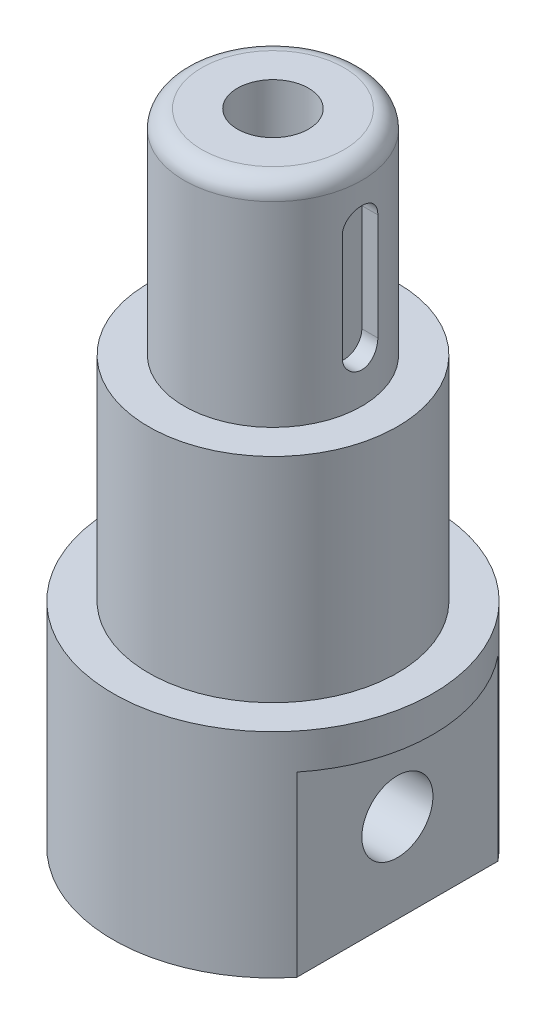
ISO-10303-21;
HEADER;
FILE_DESCRIPTION(('STEP AP214'),'2;1');
FILE_NAME('part.step','',(''),(''),'','','');
FILE_SCHEMA(('AUTOMOTIVE_DESIGN { 1 0 10303 214 1 1 1 1 }'));
ENDSEC;
DATA;
#1=APPLICATION_CONTEXT('core data for automotive mechanical design processes');
#2=APPLICATION_PROTOCOL_DEFINITION('international standard','automotive_design',2000,#1);
#3=PRODUCT_CONTEXT('',#1,'mechanical');
#4=PRODUCT('Part','Part','',(#3));
#5=PRODUCT_RELATED_PRODUCT_CATEGORY('part','',(#4));
#6=PRODUCT_DEFINITION_FORMATION('','',#4);
#7=PRODUCT_DEFINITION_CONTEXT('part definition',#1,'design');
#8=PRODUCT_DEFINITION('design','',#6,#7);
#9=PRODUCT_DEFINITION_SHAPE('','',#8);
#10=(LENGTH_UNIT() NAMED_UNIT(*) SI_UNIT(.MILLI.,.METRE.));
#11=(NAMED_UNIT(*) PLANE_ANGLE_UNIT() SI_UNIT($,.RADIAN.));
#12=(NAMED_UNIT(*) SI_UNIT($,.STERADIAN.) SOLID_ANGLE_UNIT());
#13=UNCERTAINTY_MEASURE_WITH_UNIT(LENGTH_MEASURE(1.E-05),#10,'distance_accuracy_value','');
#14=(GEOMETRIC_REPRESENTATION_CONTEXT(3) GLOBAL_UNCERTAINTY_ASSIGNED_CONTEXT((#13)) GLOBAL_UNIT_ASSIGNED_CONTEXT((#10,
#11,#12)) REPRESENTATION_CONTEXT('',''));
#15=CARTESIAN_POINT('',(0.,0.,0.));
#16=DIRECTION('',(0.,0.,1.));
#17=DIRECTION('',(1.,0.,0.));
#18=AXIS2_PLACEMENT_3D('',#15,#16,#17);
#19=CARTESIAN_POINT('',(0.,-40.6315789473685,0.));
#20=DIRECTION('',(0.,-1.,0.));
#21=DIRECTION('',(0.,0.,-1.));
#22=AXIS2_PLACEMENT_3D('',#19,#20,#21);
#23=CYLINDRICAL_SURFACE('',#22,9.99999999999998);
#24=CARTESIAN_POINT('',(-9.79795897113269,53.5481247085623,-2.));
#25=CARTESIAN_POINT('',(-9.79795611157837,53.4924575712637,-2.00000029709046));
#26=CARTESIAN_POINT('',(-9.7984339846543,53.4368176697574,-1.99767440405642));
#27=CARTESIAN_POINT('',(-9.8003213815013,53.3259472728948,-1.98839986829158));
#28=CARTESIAN_POINT('',(-9.80173079002195,53.2707167277472,-1.98145179742019));
#29=CARTESIAN_POINT('',(-9.80730283285148,53.1064148282608,-1.95376239954904));
#30=CARTESIAN_POINT('',(-9.81280956758552,52.9984618510279,-1.92617555297558));
#31=CARTESIAN_POINT('',(-9.82677660401679,52.7888395150785,-1.85359362042638));
#32=CARTESIAN_POINT('',(-9.83523723174862,52.6871708514489,-1.80859661275257));
#33=CARTESIAN_POINT('',(-9.85415440257655,52.4927949408026,-1.7025082088197));
#34=CARTESIAN_POINT('',(-9.86461115250624,52.4000886239446,-1.64141514447461));
#35=CARTESIAN_POINT('',(-9.88650550448303,52.2250050351923,-1.50396101869286));
#36=CARTESIAN_POINT('',(-9.89795377776162,52.1427721441036,-1.42741780364327));
#37=CARTESIAN_POINT('',(-9.92044851228357,51.9922158299872,-1.26162118198369));
#38=CARTESIAN_POINT('',(-9.9314949110525,51.9238945621014,-1.17236580968336));
#39=CARTESIAN_POINT('',(-9.9520562085508,51.8025469067149,-0.982720106800588));
#40=CARTESIAN_POINT('',(-9.96155694564012,51.7496587701377,-0.882239649549983));
#41=CARTESIAN_POINT('',(-9.97783510908993,51.6615729394628,-0.673602404217795));
#42=CARTESIAN_POINT('',(-9.98461293824418,51.6263726286505,-0.565446754297826));
#43=CARTESIAN_POINT('',(-9.99460635553982,51.5751106116245,-0.346034817774202));
#44=CARTESIAN_POINT('',(-9.99786765043074,51.5588031295946,-0.234838069151994));
#45=CARTESIAN_POINT('',(-10.0006184349224,51.5450227496855,-0.0112397534982628));
#46=CARTESIAN_POINT('',(-10.000108200481,51.5475484738055,0.101161724783846));
#47=CARTESIAN_POINT('',(-9.99540868887642,51.5711771093056,0.322284405513384));
#48=CARTESIAN_POINT('',(-9.99127193663418,51.5920148083719,0.43103522671446));
#49=CARTESIAN_POINT('',(-9.97984349003514,51.6512550625144,0.643464013108169));
#50=CARTESIAN_POINT('',(-9.97255169250399,51.6896581920068,0.747141812282547));
#51=CARTESIAN_POINT('',(-9.95554578241049,51.783185515553,0.94724054262592));
#52=CARTESIAN_POINT('',(-9.94581664782191,51.8384138824143,1.04361145363295));
#53=CARTESIAN_POINT('',(-9.92500903258343,51.9639452491157,1.22581287576612));
#54=CARTESIAN_POINT('',(-9.91393044014084,52.0342494982499,1.31164251244036));
#55=CARTESIAN_POINT('',(-9.89142074737008,52.1893814318128,1.47189241307715));
#56=CARTESIAN_POINT('',(-9.87998686483478,52.2744395127055,1.54608938999209));
#57=CARTESIAN_POINT('',(-9.85823412232846,52.4559342255401,1.6792217997989));
#58=CARTESIAN_POINT('',(-9.84791557170813,52.5523739988948,1.73815300484306));
#59=CARTESIAN_POINT('',(-9.82955460084641,52.7542295184542,1.83915990928954));
#60=CARTESIAN_POINT('',(-9.82151838996689,52.8596687553555,1.881189753269));
#61=CARTESIAN_POINT('',(-9.80872322124985,53.0762419710737,1.94681419465983));
#62=CARTESIAN_POINT('',(-9.80395938256573,53.1873672018586,1.97043625496866));
#63=CARTESIAN_POINT('',(-9.80006354383924,53.3408383422552,1.98966587624394));
#64=CARTESIAN_POINT('',(-9.79927519743984,53.3822329881272,1.99354251131102));
#65=CARTESIAN_POINT('',(-9.79822334773542,53.4651204368372,1.9987063293293));
#66=CARTESIAN_POINT('',(-9.79795896609648,53.5066129584739,1.99999784580931));
#67=CARTESIAN_POINT('',(-9.7979589711327,53.5481247085623,2.));
#68=B_SPLINE_CURVE_WITH_KNOTS('',3,(#24,#25,#26,#27,#28,#29,#30,#31,#32,#33,#34,#35,#36,#37,#38,
#39,#40,#41,#42,#43,#44,#45,#46,#47,#48,#49,#50,#51,#52,#53,#54,#55,#56,#57,#58,#59,#60,#61,#62,
#63,#64,#65,#66,#67),.UNSPECIFIED.,.F.,.F.,(4,2,2,2,2,2,2,2,2,2,2,2,2,2,2,2,2,2,2,2,2,4),(0.,
0.166897020715838,0.333773396643063,0.666722601037227,0.999708566174147,1.33272905329864,
1.66993288931439,2.00718892413592,2.34737937755194,2.68751948879679,3.02318320738907,
3.35882236614863,3.68967912555438,4.0205467052512,4.35350597112352,4.68649283901808,
5.02524540329293,5.3640916848566,5.70385119298729,6.04310283225105,6.16778801087552,
6.29226399953898),.UNSPECIFIED.);
#69=CARTESIAN_POINT('',(-9.79795897113269,53.5481247085623,-2.));
#70=VERTEX_POINT('',#69);
#71=CARTESIAN_POINT('',(-9.79795897113269,53.5481247085623,2.));
#72=VERTEX_POINT('',#71);
#73=EDGE_CURVE('E294',#70,#72,#68,.T.);
#74=ORIENTED_EDGE('',*,*,#73,.F.);
#75=DIRECTION('',(0.,-1.,0.));
#76=VECTOR('',#75,1.);
#77=CARTESIAN_POINT('',(-9.79795897113269,-40.6315789473685,-2.00000000000002));
#78=LINE('',#77,#76);
#79=CARTESIAN_POINT('',(-9.79795897113269,65.5481247085623,-2.));
#80=VERTEX_POINT('',#79);
#81=EDGE_CURVE('E11',#80,#70,#78,.T.);
#82=ORIENTED_EDGE('',*,*,#81,.F.);
#83=CARTESIAN_POINT('',(-9.79795897113269,65.5481247085623,2.));
#84=CARTESIAN_POINT('',(-9.79795611157837,65.603791845861,2.00000029709046));
#85=CARTESIAN_POINT('',(-9.7984339846543,65.6594317473673,1.99767440405642));
#86=CARTESIAN_POINT('',(-9.8003213815013,65.7703021442299,1.98839986829158));
#87=CARTESIAN_POINT('',(-9.80173079002195,65.8255326893775,1.98145179742019));
#88=CARTESIAN_POINT('',(-9.80730283285148,65.9898345888639,1.95376239954903));
#89=CARTESIAN_POINT('',(-9.81280956758552,66.0977875660968,1.92617555297558));
#90=CARTESIAN_POINT('',(-9.82677660401679,66.3074099020462,1.85359362042638));
#91=CARTESIAN_POINT('',(-9.83523723174862,66.4090785656758,1.80859661275257));
#92=CARTESIAN_POINT('',(-9.85415440257655,66.6034544763221,1.7025082088197));
#93=CARTESIAN_POINT('',(-9.86461115250624,66.6961607931801,1.64141514447462));
#94=CARTESIAN_POINT('',(-9.88650550448302,66.8712443819324,1.50396101869286));
#95=CARTESIAN_POINT('',(-9.89795377776162,66.9534772730211,1.42741780364328));
#96=CARTESIAN_POINT('',(-9.92044851228357,67.1040335871375,1.2616211819837));
#97=CARTESIAN_POINT('',(-9.9314949110525,67.1723548550233,1.17236580968335));
#98=CARTESIAN_POINT('',(-9.9520562085508,67.2937025104098,0.982720106800582));
#99=CARTESIAN_POINT('',(-9.96155694564012,67.346590646987,0.882239649549978));
#100=CARTESIAN_POINT('',(-9.97783510908993,67.4346764776619,0.673602404217792));
#101=CARTESIAN_POINT('',(-9.98461293824418,67.4698767884742,0.565446754297823));
#102=CARTESIAN_POINT('',(-9.99460635553982,67.5211388055002,0.3460348177742));
#103=CARTESIAN_POINT('',(-9.99786765043074,67.5374462875301,0.234838069151992));
#104=CARTESIAN_POINT('',(-10.0006184349224,67.5512266674392,0.0112397534982605));
#105=CARTESIAN_POINT('',(-10.000108200481,67.5487009433192,-0.101161724783848));
#106=CARTESIAN_POINT('',(-9.99540868887642,67.5250723078191,-0.322284405513386));
#107=CARTESIAN_POINT('',(-9.99127193663418,67.5042346087528,-0.431035226714461));
#108=CARTESIAN_POINT('',(-9.97984349003514,67.4449943546103,-0.643464013108169));
#109=CARTESIAN_POINT('',(-9.97255169250399,67.4065912251179,-0.747141812282548));
#110=CARTESIAN_POINT('',(-9.95554578241049,67.3130639015717,-0.947240542625918));
#111=CARTESIAN_POINT('',(-9.94581664782191,67.2578355347104,-1.04361145363294));
#112=CARTESIAN_POINT('',(-9.92500903258343,67.132304168009,-1.22581287576612));
#113=CARTESIAN_POINT('',(-9.91393044014084,67.0619999188748,-1.31164251244036));
#114=CARTESIAN_POINT('',(-9.89142074737008,66.9068679853119,-1.47189241307715));
#115=CARTESIAN_POINT('',(-9.87998686483478,66.8218099044192,-1.54608938999208));
#116=CARTESIAN_POINT('',(-9.85823412232846,66.6403151915846,-1.6792217997989));
#117=CARTESIAN_POINT('',(-9.84791557170813,66.5438754182299,-1.73815300484306));
#118=CARTESIAN_POINT('',(-9.82955460084641,66.3420198986705,-1.83915990928954));
#119=CARTESIAN_POINT('',(-9.82151838996689,66.2365806617692,-1.881189753269));
#120=CARTESIAN_POINT('',(-9.80872322124985,66.020007446051,-1.94681419465982));
#121=CARTESIAN_POINT('',(-9.80395938256573,65.9088822152661,-1.97043625496865));
#122=CARTESIAN_POINT('',(-9.80006354383924,65.7554110748695,-1.98966587624393));
#123=CARTESIAN_POINT('',(-9.79927519743984,65.7140164289975,-1.99354251131102));
#124=CARTESIAN_POINT('',(-9.79822334773542,65.6311289802875,-1.9987063293293));
#125=CARTESIAN_POINT('',(-9.79795896609648,65.5896364586508,-1.99999784580931));
#126=CARTESIAN_POINT('',(-9.7979589711327,65.5481247085624,-2.));
#127=B_SPLINE_CURVE_WITH_KNOTS('',3,(#83,#84,#85,#86,#87,#88,#89,#90,#91,#92,#93,#94,#95,#96,
#97,#98,#99,#100,#101,#102,#103,#104,#105,#106,#107,#108,#109,#110,#111,#112,#113,#114,#115,
#116,#117,#118,#119,#120,#121,#122,#123,#124,#125,#126),.UNSPECIFIED.,.F.,.F.,(4,2,2,2,2,2,2,2,
2,2,2,2,2,2,2,2,2,2,2,2,2,4),(0.,0.166897020715817,0.333773396643063,0.666722601037227,
0.999708566174146,1.33272905329863,1.66993288931438,2.00718892413592,2.34737937755194,
2.68751948879679,3.02318320738908,3.35882236614863,3.68967912555438,4.02054670525121,
4.35350597112352,4.68649283901807,5.02524540329292,5.3640916848566,5.70385119298727,
6.04310283225103,6.16778801087547,6.29226399953897),.UNSPECIFIED.);
#128=CARTESIAN_POINT('',(-9.79795897113269,65.5481247085623,2.));
#129=VERTEX_POINT('',#128);
#130=EDGE_CURVE('E142',#129,#80,#127,.T.);
#131=ORIENTED_EDGE('',*,*,#130,.F.);
#132=DIRECTION('',(0.,-1.,0.));
#133=VECTOR('',#132,1.);
#134=CARTESIAN_POINT('',(-9.79795897113269,-40.6315789473685,2.00000000000001));
#135=LINE('',#134,#133);
#136=EDGE_CURVE('E50',#72,#129,#135,.F.);
#137=ORIENTED_EDGE('',*,*,#136,.F.);
#138=EDGE_LOOP('',(#74,#82,#131,#137));
#139=FACE_BOUND('',#138,.T.);
#140=CARTESIAN_POINT('',(0.,70.,0.));
#141=DIRECTION('',(0.,1.,0.));
#142=DIRECTION('',(0.,0.,1.));
#143=AXIS2_PLACEMENT_3D('',#140,#141,#142);
#144=CIRCLE('',#143,9.99999999999998);
#145=CARTESIAN_POINT('',(0.,70.,9.99999999999998));
#146=VERTEX_POINT('',#145);
#147=EDGE_CURVE('E246',#146,#146,#144,.F.);
#148=ORIENTED_EDGE('',*,*,#147,.T.);
#149=EDGE_LOOP('',(#148));
#150=FACE_BOUND('',#149,.T.);
#151=CARTESIAN_POINT('',(0.,48.,0.));
#152=DIRECTION('',(0.,-1.,0.));
#153=DIRECTION('',(0.,0.,-1.));
#154=AXIS2_PLACEMENT_3D('',#151,#152,#153);
#155=CIRCLE('',#154,9.99999999999998);
#156=CARTESIAN_POINT('',(0.,48.,-9.99999999999998));
#157=VERTEX_POINT('',#156);
#158=EDGE_CURVE('E212',#157,#157,#155,.T.);
#159=ORIENTED_EDGE('',*,*,#158,.F.);
#160=EDGE_LOOP('',(#159));
#161=FACE_BOUND('',#160,.T.);
#162=DIRECTION('',(0.,-1.,0.));
#163=VECTOR('',#162,1.);
#164=CARTESIAN_POINT('',(9.79795897113269,-40.6315789473685,-2.00000000000002));
#165=LINE('',#164,#163);
#166=CARTESIAN_POINT('',(9.79795897113269,65.5481247085623,-2.));
#167=VERTEX_POINT('',#166);
#168=CARTESIAN_POINT('',(9.79795897113269,53.5481247085624,-2.00000000000002));
#169=VERTEX_POINT('',#168);
#170=EDGE_CURVE('E292',#167,#169,#165,.T.);
#171=ORIENTED_EDGE('',*,*,#170,.T.);
#172=CARTESIAN_POINT('',(9.79795897113269,53.5481247085623,-2.));
#173=CARTESIAN_POINT('',(9.79795611157837,53.4924575712637,-2.00000029709046));
#174=CARTESIAN_POINT('',(9.7984339846543,53.4368176697574,-1.99767440405642));
#175=CARTESIAN_POINT('',(9.8003213815013,53.3259472728948,-1.98839986829158));
#176=CARTESIAN_POINT('',(9.80173079002195,53.2707167277472,-1.98145179742019));
#177=CARTESIAN_POINT('',(9.80730283285148,53.1064148282608,-1.95376239954904));
#178=CARTESIAN_POINT('',(9.81280956758552,52.9984618510279,-1.92617555297558));
#179=CARTESIAN_POINT('',(9.82677660401679,52.7888395150785,-1.85359362042638));
#180=CARTESIAN_POINT('',(9.83523723174862,52.6871708514489,-1.80859661275257));
#181=CARTESIAN_POINT('',(9.85415440257655,52.4927949408026,-1.7025082088197));
#182=CARTESIAN_POINT('',(9.86461115250624,52.4000886239446,-1.64141514447461));
#183=CARTESIAN_POINT('',(9.88650550448303,52.2250050351923,-1.50396101869286));
#184=CARTESIAN_POINT('',(9.89795377776162,52.1427721441036,-1.42741780364327));
#185=CARTESIAN_POINT('',(9.92044851228357,51.9922158299872,-1.26162118198369));
#186=CARTESIAN_POINT('',(9.9314949110525,51.9238945621014,-1.17236580968336));
#187=CARTESIAN_POINT('',(9.9520562085508,51.8025469067149,-0.982720106800588));
#188=CARTESIAN_POINT('',(9.96155694564012,51.7496587701377,-0.882239649549983));
#189=CARTESIAN_POINT('',(9.97783510908993,51.6615729394628,-0.673602404217795));
#190=CARTESIAN_POINT('',(9.98461293824418,51.6263726286505,-0.565446754297826));
#191=CARTESIAN_POINT('',(9.99460635553982,51.5751106116245,-0.346034817774202));
#192=CARTESIAN_POINT('',(9.99786765043074,51.5588031295946,-0.234838069151994));
#193=CARTESIAN_POINT('',(10.0006184349224,51.5450227496855,-0.0112397534982628));
#194=CARTESIAN_POINT('',(10.000108200481,51.5475484738055,0.101161724783846));
#195=CARTESIAN_POINT('',(9.99540868887642,51.5711771093056,0.322284405513384));
#196=CARTESIAN_POINT('',(9.99127193663418,51.5920148083719,0.43103522671446));
#197=CARTESIAN_POINT('',(9.97984349003514,51.6512550625144,0.643464013108169));
#198=CARTESIAN_POINT('',(9.97255169250399,51.6896581920068,0.747141812282547));
#199=CARTESIAN_POINT('',(9.95554578241049,51.783185515553,0.94724054262592));
#200=CARTESIAN_POINT('',(9.94581664782191,51.8384138824143,1.04361145363295));
#201=CARTESIAN_POINT('',(9.92500903258343,51.9639452491157,1.22581287576612));
#202=CARTESIAN_POINT('',(9.91393044014084,52.0342494982499,1.31164251244036));
#203=CARTESIAN_POINT('',(9.89142074737008,52.1893814318128,1.47189241307715));
#204=CARTESIAN_POINT('',(9.87998686483478,52.2744395127055,1.54608938999209));
#205=CARTESIAN_POINT('',(9.85823412232846,52.4559342255401,1.6792217997989));
#206=CARTESIAN_POINT('',(9.84791557170813,52.5523739988948,1.73815300484306));
#207=CARTESIAN_POINT('',(9.82955460084641,52.7542295184542,1.83915990928954));
#208=CARTESIAN_POINT('',(9.82151838996689,52.8596687553555,1.881189753269));
#209=CARTESIAN_POINT('',(9.80872322124985,53.0762419710737,1.94681419465983));
#210=CARTESIAN_POINT('',(9.80395938256573,53.1873672018586,1.97043625496866));
#211=CARTESIAN_POINT('',(9.80006354383924,53.3408383422552,1.98966587624394));
#212=CARTESIAN_POINT('',(9.79927519743984,53.3822329881272,1.99354251131102));
#213=CARTESIAN_POINT('',(9.79822334773542,53.4651204368372,1.9987063293293));
#214=CARTESIAN_POINT('',(9.79795896609648,53.5066129584739,1.99999784580931));
#215=CARTESIAN_POINT('',(9.7979589711327,53.5481247085623,2.));
#216=B_SPLINE_CURVE_WITH_KNOTS('',3,(#172,#173,#174,#175,#176,#177,#178,#179,#180,#181,#182,
#183,#184,#185,#186,#187,#188,#189,#190,#191,#192,#193,#194,#195,#196,#197,#198,#199,#200,#201,
#202,#203,#204,#205,#206,#207,#208,#209,#210,#211,#212,#213,#214,#215),.UNSPECIFIED.,.F.,.F.,(4,
2,2,2,2,2,2,2,2,2,2,2,2,2,2,2,2,2,2,2,2,4),(0.,0.166897020715838,0.333773396643063,
0.666722601037227,0.999708566174147,1.33272905329864,1.66993288931439,2.00718892413592,
2.34737937755194,2.68751948879679,3.02318320738907,3.35882236614863,3.68967912555438,
4.0205467052512,4.35350597112352,4.68649283901808,5.02524540329293,5.3640916848566,
5.70385119298729,6.04310283225105,6.16778801087552,6.29226399953898),.UNSPECIFIED.);
#217=CARTESIAN_POINT('',(9.79795897113269,53.5481247085623,2.));
#218=VERTEX_POINT('',#217);
#219=EDGE_CURVE('E65',#169,#218,#216,.T.);
#220=ORIENTED_EDGE('',*,*,#219,.T.);
#221=DIRECTION('',(0.,-1.,0.));
#222=VECTOR('',#221,1.);
#223=CARTESIAN_POINT('',(9.79795897113269,-40.6315789473685,2.00000000000001));
#224=LINE('',#223,#222);
#225=CARTESIAN_POINT('',(9.79795897113269,65.5481247085623,2.));
#226=VERTEX_POINT('',#225);
#227=EDGE_CURVE('E261',#218,#226,#224,.F.);
#228=ORIENTED_EDGE('',*,*,#227,.T.);
#229=CARTESIAN_POINT('',(9.79795897113269,65.5481247085623,2.));
#230=CARTESIAN_POINT('',(9.79795611157837,65.603791845861,2.00000029709046));
#231=CARTESIAN_POINT('',(9.7984339846543,65.6594317473673,1.99767440405642));
#232=CARTESIAN_POINT('',(9.8003213815013,65.7703021442299,1.98839986829158));
#233=CARTESIAN_POINT('',(9.80173079002195,65.8255326893775,1.98145179742019));
#234=CARTESIAN_POINT('',(9.80730283285148,65.9898345888639,1.95376239954903));
#235=CARTESIAN_POINT('',(9.81280956758552,66.0977875660968,1.92617555297558));
#236=CARTESIAN_POINT('',(9.82677660401679,66.3074099020462,1.85359362042638));
#237=CARTESIAN_POINT('',(9.83523723174862,66.4090785656758,1.80859661275257));
#238=CARTESIAN_POINT('',(9.85415440257655,66.6034544763221,1.7025082088197));
#239=CARTESIAN_POINT('',(9.86461115250624,66.6961607931801,1.64141514447462));
#240=CARTESIAN_POINT('',(9.88650550448302,66.8712443819324,1.50396101869286));
#241=CARTESIAN_POINT('',(9.89795377776162,66.9534772730211,1.42741780364328));
#242=CARTESIAN_POINT('',(9.92044851228357,67.1040335871375,1.2616211819837));
#243=CARTESIAN_POINT('',(9.9314949110525,67.1723548550233,1.17236580968335));
#244=CARTESIAN_POINT('',(9.9520562085508,67.2937025104098,0.982720106800582));
#245=CARTESIAN_POINT('',(9.96155694564012,67.346590646987,0.882239649549978));
#246=CARTESIAN_POINT('',(9.97783510908993,67.4346764776619,0.673602404217792));
#247=CARTESIAN_POINT('',(9.98461293824418,67.4698767884742,0.565446754297823));
#248=CARTESIAN_POINT('',(9.99460635553982,67.5211388055002,0.3460348177742));
#249=CARTESIAN_POINT('',(9.99786765043074,67.5374462875301,0.234838069151992));
#250=CARTESIAN_POINT('',(10.0006184349224,67.5512266674392,0.0112397534982605));
#251=CARTESIAN_POINT('',(10.000108200481,67.5487009433192,-0.101161724783848));
#252=CARTESIAN_POINT('',(9.99540868887642,67.5250723078191,-0.322284405513386));
#253=CARTESIAN_POINT('',(9.99127193663418,67.5042346087528,-0.431035226714461));
#254=CARTESIAN_POINT('',(9.97984349003514,67.4449943546103,-0.643464013108169));
#255=CARTESIAN_POINT('',(9.97255169250399,67.4065912251179,-0.747141812282548));
#256=CARTESIAN_POINT('',(9.95554578241049,67.3130639015717,-0.947240542625918));
#257=CARTESIAN_POINT('',(9.94581664782191,67.2578355347104,-1.04361145363294));
#258=CARTESIAN_POINT('',(9.92500903258343,67.132304168009,-1.22581287576612));
#259=CARTESIAN_POINT('',(9.91393044014084,67.0619999188748,-1.31164251244036));
#260=CARTESIAN_POINT('',(9.89142074737008,66.9068679853119,-1.47189241307715));
#261=CARTESIAN_POINT('',(9.87998686483478,66.8218099044192,-1.54608938999208));
#262=CARTESIAN_POINT('',(9.85823412232846,66.6403151915846,-1.6792217997989));
#263=CARTESIAN_POINT('',(9.84791557170813,66.5438754182299,-1.73815300484306));
#264=CARTESIAN_POINT('',(9.82955460084641,66.3420198986705,-1.83915990928954));
#265=CARTESIAN_POINT('',(9.82151838996689,66.2365806617692,-1.881189753269));
#266=CARTESIAN_POINT('',(9.80872322124985,66.020007446051,-1.94681419465982));
#267=CARTESIAN_POINT('',(9.80395938256573,65.9088822152661,-1.97043625496865));
#268=CARTESIAN_POINT('',(9.80006354383924,65.7554110748695,-1.98966587624393));
#269=CARTESIAN_POINT('',(9.79927519743984,65.7140164289975,-1.99354251131102));
#270=CARTESIAN_POINT('',(9.79822334773542,65.6311289802875,-1.9987063293293));
#271=CARTESIAN_POINT('',(9.79795896609648,65.5896364586508,-1.99999784580931));
#272=CARTESIAN_POINT('',(9.7979589711327,65.5481247085624,-2.));
#273=B_SPLINE_CURVE_WITH_KNOTS('',3,(#229,#230,#231,#232,#233,#234,#235,#236,#237,#238,#239,
#240,#241,#242,#243,#244,#245,#246,#247,#248,#249,#250,#251,#252,#253,#254,#255,#256,#257,#258,
#259,#260,#261,#262,#263,#264,#265,#266,#267,#268,#269,#270,#271,#272),.UNSPECIFIED.,.F.,.F.,(4,
2,2,2,2,2,2,2,2,2,2,2,2,2,2,2,2,2,2,2,2,4),(0.,0.166897020715817,0.333773396643063,
0.666722601037227,0.999708566174146,1.33272905329863,1.66993288931438,2.00718892413592,
2.34737937755194,2.68751948879679,3.02318320738908,3.35882236614863,3.68967912555438,
4.02054670525121,4.35350597112352,4.68649283901807,5.02524540329292,5.3640916848566,
5.70385119298727,6.04310283225103,6.16778801087547,6.29226399953897),.UNSPECIFIED.);
#274=EDGE_CURVE('E284',#226,#167,#273,.T.);
#275=ORIENTED_EDGE('',*,*,#274,.T.);
#276=EDGE_LOOP('',(#171,#220,#228,#275));
#277=FACE_BOUND('',#276,.T.);
#278=ADVANCED_FACE('F39',(#139,#150,#161,#277),#23,.T.);
#279=CARTESIAN_POINT('',(0.,-40.6315789473685,0.));
#280=DIRECTION('',(0.,-1.,0.));
#281=DIRECTION('',(0.,0.,-1.));
#282=AXIS2_PLACEMENT_3D('',#279,#280,#281);
#283=CYLINDRICAL_SURFACE('',#282,4.);
#284=CARTESIAN_POINT('',(0.,10.,0.));
#285=DIRECTION('',(-0.707106781186547,-0.707106781186547,0.));
#286=DIRECTION('',(0.707106781186547,-0.707106781186547,0.));
#287=AXIS2_PLACEMENT_3D('',#284,#285,#286);
#288=ELLIPSE('',#287,5.65685424949238,4.);
#289=CARTESIAN_POINT('',(0.,10.,-4.));
#290=VERTEX_POINT('',#289);
#291=CARTESIAN_POINT('',(0.,10.,4.));
#292=VERTEX_POINT('',#291);
#293=EDGE_CURVE('E200',#290,#292,#288,.F.);
#294=ORIENTED_EDGE('',*,*,#293,.F.);
#295=CARTESIAN_POINT('',(0.,10.,0.));
#296=DIRECTION('',(0.707106781186547,-0.707106781186547,0.));
#297=DIRECTION('',(-0.707106781186547,-0.707106781186547,0.));
#298=AXIS2_PLACEMENT_3D('',#295,#296,#297);
#299=ELLIPSE('',#298,5.65685424949238,4.);
#300=EDGE_CURVE('E191',#292,#290,#299,.F.);
#301=ORIENTED_EDGE('',*,*,#300,.F.);
#302=EDGE_LOOP('',(#294,#301));
#303=FACE_BOUND('',#302,.T.);
#304=CARTESIAN_POINT('',(0.,72.,0.));
#305=DIRECTION('',(0.,-1.,0.));
#306=DIRECTION('',(0.,0.,-1.));
#307=AXIS2_PLACEMENT_3D('',#304,#305,#306);
#308=CIRCLE('',#307,4.);
#309=CARTESIAN_POINT('',(0.,72.,-4.));
#310=VERTEX_POINT('',#309);
#311=EDGE_CURVE('E243',#310,#310,#308,.T.);
#312=ORIENTED_EDGE('',*,*,#311,.F.);
#313=EDGE_LOOP('',(#312));
#314=FACE_BOUND('',#313,.T.);
#315=ADVANCED_FACE('F324',(#303,#314),#283,.F.);
#316=CARTESIAN_POINT('',(9.99999999999998,72.,0.));
#317=DIRECTION('',(0.,1.,0.));
#318=DIRECTION('',(0.,0.,1.));
#319=AXIS2_PLACEMENT_3D('',#316,#317,#318);
#320=PLANE('',#319);
#321=CARTESIAN_POINT('',(0.,72.,0.));
#322=DIRECTION('',(0.,1.,0.));
#323=DIRECTION('',(0.,0.,1.));
#324=AXIS2_PLACEMENT_3D('',#321,#322,#323);
#325=CIRCLE('',#324,7.99999999999998);
#326=CARTESIAN_POINT('',(0.,72.,7.99999999999998));
#327=VERTEX_POINT('',#326);
#328=EDGE_CURVE('E253',#327,#327,#325,.T.);
#329=ORIENTED_EDGE('',*,*,#328,.T.);
#330=EDGE_LOOP('',(#329));
#331=FACE_BOUND('',#330,.T.);
#332=ORIENTED_EDGE('',*,*,#311,.T.);
#333=EDGE_LOOP('',(#332));
#334=FACE_BOUND('',#333,.T.);
#335=ADVANCED_FACE('F329',(#331,#334),#320,.T.);
#336=CARTESIAN_POINT('',(0.,10.,0.));
#337=DIRECTION('',(-0.707106781186547,-0.707106781186547,0.));
#338=DIRECTION('',(0.707106781186547,-0.707106781186547,0.));
#339=AXIS2_PLACEMENT_3D('',#336,#337,#338);
#340=ELLIPSE('',#339,5.65685424949238,4.);
#341=EDGE_CURVE('E198',#290,#292,#340,.T.);
#342=ORIENTED_EDGE('',*,*,#341,.F.);
#343=CARTESIAN_POINT('',(0.,10.,0.));
#344=DIRECTION('',(0.707106781186547,-0.707106781186547,0.));
#345=DIRECTION('',(-0.707106781186547,-0.707106781186547,0.));
#346=AXIS2_PLACEMENT_3D('',#343,#344,#345);
#347=ELLIPSE('',#346,5.65685424949238,4.);
#348=EDGE_CURVE('E192',#292,#290,#347,.T.);
#349=ORIENTED_EDGE('',*,*,#348,.F.);
#350=EDGE_LOOP('',(#342,#349));
#351=FACE_BOUND('',#350,.T.);
#352=CARTESIAN_POINT('',(0.,0.,0.));
#353=DIRECTION('',(0.,-1.,0.));
#354=DIRECTION('',(0.,0.,-1.));
#355=AXIS2_PLACEMENT_3D('',#352,#353,#354);
#356=CIRCLE('',#355,4.);
#357=CARTESIAN_POINT('',(0.,0.,-4.));
#358=VERTEX_POINT('',#357);
#359=EDGE_CURVE('E238',#358,#358,#356,.T.);
#360=ORIENTED_EDGE('',*,*,#359,.T.);
#361=EDGE_LOOP('',(#360));
#362=FACE_BOUND('',#361,.T.);
#363=ADVANCED_FACE('F334',(#351,#362),#283,.F.);
#364=CARTESIAN_POINT('',(4.,0.,0.));
#365=DIRECTION('',(0.,-1.,0.));
#366=DIRECTION('',(0.,0.,-1.));
#367=AXIS2_PLACEMENT_3D('',#364,#365,#366);
#368=PLANE('',#367);
#369=DIRECTION('',(0.,0.,-1.));
#370=VECTOR('',#369,1.);
#371=CARTESIAN_POINT('',(14.,0.,11.3137084989848));
#372=LINE('',#371,#370);
#373=CARTESIAN_POINT('',(14.,0.,11.3137084989848));
#374=VERTEX_POINT('',#373);
#375=CARTESIAN_POINT('',(14.,0.,-11.3137084989848));
#376=VERTEX_POINT('',#375);
#377=EDGE_CURVE('E206',#374,#376,#372,.T.);
#378=ORIENTED_EDGE('',*,*,#377,.F.);
#379=CARTESIAN_POINT('',(0.,0.,0.));
#380=DIRECTION('',(0.,-1.,0.));
#381=DIRECTION('',(0.,0.,-1.));
#382=AXIS2_PLACEMENT_3D('',#379,#380,#381);
#383=CIRCLE('',#382,18.);
#384=CARTESIAN_POINT('',(-14.,0.,11.3137084989848));
#385=VERTEX_POINT('',#384);
#386=EDGE_CURVE('E239',#374,#385,#383,.T.);
#387=ORIENTED_EDGE('',*,*,#386,.T.);
#388=DIRECTION('',(0.,0.,1.));
#389=VECTOR('',#388,1.);
#390=CARTESIAN_POINT('',(-14.,0.,11.3137084989848));
#391=LINE('',#390,#389);
#392=CARTESIAN_POINT('',(-14.,0.,-11.3137084989848));
#393=VERTEX_POINT('',#392);
#394=EDGE_CURVE('E205',#393,#385,#391,.T.);
#395=ORIENTED_EDGE('',*,*,#394,.F.);
#396=EDGE_CURVE('E237',#393,#376,#383,.T.);
#397=ORIENTED_EDGE('',*,*,#396,.T.);
#398=EDGE_LOOP('',(#378,#387,#395,#397));
#399=FACE_BOUND('',#398,.T.);
#400=ORIENTED_EDGE('',*,*,#359,.F.);
#401=EDGE_LOOP('',(#400));
#402=FACE_BOUND('',#401,.T.);
#403=ADVANCED_FACE('F366',(#399,#402),#368,.T.);
#404=CARTESIAN_POINT('',(0.,-40.6315789473685,0.));
#405=DIRECTION('',(0.,-1.,0.));
#406=DIRECTION('',(0.,0.,-1.));
#407=AXIS2_PLACEMENT_3D('',#404,#405,#406);
#408=CYLINDRICAL_SURFACE('',#407,18.);
#409=DIRECTION('',(0.,-1.,0.));
#410=VECTOR('',#409,1.);
#411=CARTESIAN_POINT('',(14.,20.,-11.3137084989848));
#412=LINE('',#411,#410);
#413=CARTESIAN_POINT('',(14.,20.,-11.3137084989848));
#414=VERTEX_POINT('',#413);
#415=EDGE_CURVE('E211',#414,#376,#412,.T.);
#416=ORIENTED_EDGE('',*,*,#415,.T.);
#417=ORIENTED_EDGE('',*,*,#396,.F.);
#418=DIRECTION('',(0.,-1.,0.));
#419=VECTOR('',#418,1.);
#420=CARTESIAN_POINT('',(-14.,20.,-11.3137084989848));
#421=LINE('',#420,#419);
#422=CARTESIAN_POINT('',(-14.,20.,-11.3137084989848));
#423=VERTEX_POINT('',#422);
#424=EDGE_CURVE('E219',#423,#393,#421,.T.);
#425=ORIENTED_EDGE('',*,*,#424,.F.);
#426=CARTESIAN_POINT('',(0.,20.,0.));
#427=DIRECTION('',(0.,-1.,0.));
#428=DIRECTION('',(0.,0.,-1.));
#429=AXIS2_PLACEMENT_3D('',#426,#427,#428);
#430=CIRCLE('',#429,18.);
#431=CARTESIAN_POINT('',(-14.,20.,11.3137084989848));
#432=VERTEX_POINT('',#431);
#433=EDGE_CURVE('E216',#432,#423,#430,.T.);
#434=ORIENTED_EDGE('',*,*,#433,.F.);
#435=DIRECTION('',(0.,-1.,0.));
#436=VECTOR('',#435,1.);
#437=CARTESIAN_POINT('',(-14.,20.,11.3137084989848));
#438=LINE('',#437,#436);
#439=EDGE_CURVE('E209',#432,#385,#438,.T.);
#440=ORIENTED_EDGE('',*,*,#439,.T.);
#441=ORIENTED_EDGE('',*,*,#386,.F.);
#442=DIRECTION('',(0.,-1.,0.));
#443=VECTOR('',#442,1.);
#444=CARTESIAN_POINT('',(14.,20.,11.3137084989848));
#445=LINE('',#444,#443);
#446=CARTESIAN_POINT('',(14.,20.,11.3137084989848));
#447=VERTEX_POINT('',#446);
#448=EDGE_CURVE('E208',#447,#374,#445,.T.);
#449=ORIENTED_EDGE('',*,*,#448,.F.);
#450=CARTESIAN_POINT('',(0.,20.,0.));
#451=DIRECTION('',(0.,-1.,0.));
#452=DIRECTION('',(0.,0.,-1.));
#453=AXIS2_PLACEMENT_3D('',#450,#451,#452);
#454=CIRCLE('',#453,18.);
#455=EDGE_CURVE('E201',#414,#447,#454,.T.);
#456=ORIENTED_EDGE('',*,*,#455,.F.);
#457=EDGE_LOOP('',(#416,#417,#425,#434,#440,#441,#449,#456));
#458=FACE_BOUND('',#457,.T.);
#459=CARTESIAN_POINT('',(0.,24.,0.));
#460=DIRECTION('',(0.,-1.,0.));
#461=DIRECTION('',(0.,0.,-1.));
#462=AXIS2_PLACEMENT_3D('',#459,#460,#461);
#463=CIRCLE('',#462,18.);
#464=CARTESIAN_POINT('',(0.,24.,-18.));
#465=VERTEX_POINT('',#464);
#466=EDGE_CURVE('E233',#465,#465,#463,.T.);
#467=ORIENTED_EDGE('',*,*,#466,.T.);
#468=EDGE_LOOP('',(#467));
#469=FACE_BOUND('',#468,.T.);
#470=ADVANCED_FACE('F361',(#458,#469),#408,.T.);
#471=CARTESIAN_POINT('',(18.,24.,0.));
#472=DIRECTION('',(0.,1.,0.));
#473=DIRECTION('',(0.,0.,1.));
#474=AXIS2_PLACEMENT_3D('',#471,#472,#473);
#475=PLANE('',#474);
#476=CARTESIAN_POINT('',(0.,24.,0.));
#477=DIRECTION('',(0.,-1.,0.));
#478=DIRECTION('',(0.,0.,-1.));
#479=AXIS2_PLACEMENT_3D('',#476,#477,#478);
#480=CIRCLE('',#479,14.);
#481=CARTESIAN_POINT('',(0.,24.,-14.));
#482=VERTEX_POINT('',#481);
#483=EDGE_CURVE('E226',#482,#482,#480,.T.);
#484=ORIENTED_EDGE('',*,*,#483,.T.);
#485=EDGE_LOOP('',(#484));
#486=FACE_BOUND('',#485,.T.);
#487=ORIENTED_EDGE('',*,*,#466,.F.);
#488=EDGE_LOOP('',(#487));
#489=FACE_BOUND('',#488,.T.);
#490=ADVANCED_FACE('F360',(#486,#489),#475,.T.);
#491=CARTESIAN_POINT('',(0.,-40.6315789473685,0.));
#492=DIRECTION('',(0.,-1.,0.));
#493=DIRECTION('',(0.,0.,-1.));
#494=AXIS2_PLACEMENT_3D('',#491,#492,#493);
#495=CYLINDRICAL_SURFACE('',#494,14.);
#496=CARTESIAN_POINT('',(0.,48.,0.));
#497=DIRECTION('',(0.,-1.,0.));
#498=DIRECTION('',(0.,0.,-1.));
#499=AXIS2_PLACEMENT_3D('',#496,#497,#498);
#500=CIRCLE('',#499,14.);
#501=CARTESIAN_POINT('',(0.,48.,-14.));
#502=VERTEX_POINT('',#501);
#503=EDGE_CURVE('E230',#502,#502,#500,.T.);
#504=ORIENTED_EDGE('',*,*,#503,.T.);
#505=EDGE_LOOP('',(#504));
#506=FACE_BOUND('',#505,.T.);
#507=ORIENTED_EDGE('',*,*,#483,.F.);
#508=EDGE_LOOP('',(#507));
#509=FACE_BOUND('',#508,.T.);
#510=ADVANCED_FACE('F355',(#506,#509),#495,.T.);
#511=CARTESIAN_POINT('',(14.,48.,0.));
#512=DIRECTION('',(0.,1.,0.));
#513=DIRECTION('',(0.,0.,1.));
#514=AXIS2_PLACEMENT_3D('',#511,#512,#513);
#515=PLANE('',#514);
#516=ORIENTED_EDGE('',*,*,#158,.T.);
#517=EDGE_LOOP('',(#516));
#518=FACE_BOUND('',#517,.T.);
#519=ORIENTED_EDGE('',*,*,#503,.F.);
#520=EDGE_LOOP('',(#519));
#521=FACE_BOUND('',#520,.T.);
#522=ADVANCED_FACE('F346',(#518,#521),#515,.T.);
#523=CARTESIAN_POINT('',(-14.,20.,11.3137084989848));
#524=DIRECTION('',(1.,0.,0.));
#525=DIRECTION('',(0.,0.,-1.));
#526=AXIS2_PLACEMENT_3D('',#523,#524,#525);
#527=PLANE('',#526);
#528=CARTESIAN_POINT('',(-14.,10.,0.));
#529=DIRECTION('',(-1.,0.,0.));
#530=DIRECTION('',(0.,0.,1.));
#531=AXIS2_PLACEMENT_3D('',#528,#529,#530);
#532=CIRCLE('',#531,4.);
#533=CARTESIAN_POINT('',(-14.,10.,4.));
#534=VERTEX_POINT('',#533);
#535=EDGE_CURVE('E190',#534,#534,#532,.T.);
#536=ORIENTED_EDGE('',*,*,#535,.F.);
#537=EDGE_LOOP('',(#536));
#538=FACE_BOUND('',#537,.T.);
#539=ORIENTED_EDGE('',*,*,#394,.T.);
#540=ORIENTED_EDGE('',*,*,#439,.F.);
#541=DIRECTION('',(0.,0.,1.));
#542=VECTOR('',#541,1.);
#543=CARTESIAN_POINT('',(-14.,20.,11.3137084989848));
#544=LINE('',#543,#542);
#545=EDGE_CURVE('E217',#423,#432,#544,.T.);
#546=ORIENTED_EDGE('',*,*,#545,.F.);
#547=ORIENTED_EDGE('',*,*,#424,.T.);
#548=EDGE_LOOP('',(#539,#540,#546,#547));
#549=FACE_BOUND('',#548,.T.);
#550=ADVANCED_FACE('F352',(#538,#549),#527,.F.);
#551=CARTESIAN_POINT('',(0.,20.,0.));
#552=DIRECTION('',(0.,-1.,0.));
#553=DIRECTION('',(0.,0.,-1.));
#554=AXIS2_PLACEMENT_3D('',#551,#552,#553);
#555=PLANE('',#554);
#556=ORIENTED_EDGE('',*,*,#433,.T.);
#557=ORIENTED_EDGE('',*,*,#545,.T.);
#558=EDGE_LOOP('',(#556,#557));
#559=FACE_BOUND('',#558,.T.);
#560=ADVANCED_FACE('F410',(#559),#555,.T.);
#561=CARTESIAN_POINT('',(14.,20.,11.3137084989848));
#562=DIRECTION('',(-1.,0.,0.));
#563=DIRECTION('',(0.,0.,1.));
#564=AXIS2_PLACEMENT_3D('',#561,#562,#563);
#565=PLANE('',#564);
#566=CARTESIAN_POINT('',(14.,10.,0.));
#567=DIRECTION('',(-1.,0.,0.));
#568=DIRECTION('',(0.,0.,1.));
#569=AXIS2_PLACEMENT_3D('',#566,#567,#568);
#570=CIRCLE('',#569,4.);
#571=CARTESIAN_POINT('',(14.,10.,4.));
#572=VERTEX_POINT('',#571);
#573=EDGE_CURVE('E186',#572,#572,#570,.T.);
#574=ORIENTED_EDGE('',*,*,#573,.T.);
#575=EDGE_LOOP('',(#574));
#576=FACE_BOUND('',#575,.T.);
#577=ORIENTED_EDGE('',*,*,#377,.T.);
#578=ORIENTED_EDGE('',*,*,#415,.F.);
#579=DIRECTION('',(0.,0.,-1.));
#580=VECTOR('',#579,1.);
#581=CARTESIAN_POINT('',(14.,20.,11.3137084989848));
#582=LINE('',#581,#580);
#583=EDGE_CURVE('E202',#447,#414,#582,.T.);
#584=ORIENTED_EDGE('',*,*,#583,.F.);
#585=ORIENTED_EDGE('',*,*,#448,.T.);
#586=EDGE_LOOP('',(#577,#578,#584,#585));
#587=FACE_BOUND('',#586,.T.);
#588=ADVANCED_FACE('F423',(#576,#587),#565,.F.);
#589=CARTESIAN_POINT('',(0.,20.,0.));
#590=DIRECTION('',(0.,-1.,0.));
#591=DIRECTION('',(0.,0.,-1.));
#592=AXIS2_PLACEMENT_3D('',#589,#590,#591);
#593=PLANE('',#592);
#594=ORIENTED_EDGE('',*,*,#455,.T.);
#595=ORIENTED_EDGE('',*,*,#583,.T.);
#596=EDGE_LOOP('',(#594,#595));
#597=FACE_BOUND('',#596,.T.);
#598=ADVANCED_FACE('F398',(#597),#593,.T.);
#599=CARTESIAN_POINT('',(16.,10.,0.));
#600=DIRECTION('',(-1.,0.,0.));
#601=DIRECTION('',(0.,0.,1.));
#602=AXIS2_PLACEMENT_3D('',#599,#600,#601);
#603=CYLINDRICAL_SURFACE('',#602,4.);
#604=ORIENTED_EDGE('',*,*,#341,.T.);
#605=ORIENTED_EDGE('',*,*,#300,.T.);
#606=EDGE_LOOP('',(#604,#605));
#607=FACE_BOUND('',#606,.T.);
#608=ORIENTED_EDGE('',*,*,#573,.F.);
#609=EDGE_LOOP('',(#608));
#610=FACE_BOUND('',#609,.T.);
#611=ADVANCED_FACE('F285',(#607,#610),#603,.F.);
#612=ORIENTED_EDGE('',*,*,#293,.T.);
#613=ORIENTED_EDGE('',*,*,#348,.T.);
#614=EDGE_LOOP('',(#612,#613));
#615=FACE_BOUND('',#614,.T.);
#616=ORIENTED_EDGE('',*,*,#535,.T.);
#617=EDGE_LOOP('',(#616));
#618=FACE_BOUND('',#617,.T.);
#619=ADVANCED_FACE('F392',(#615,#618),#603,.F.);
#620=CARTESIAN_POINT('',(0.,70.,0.));
#621=DIRECTION('',(0.,1.,0.));
#622=DIRECTION('',(0.,0.,1.));
#623=AXIS2_PLACEMENT_3D('',#620,#621,#622);
#624=TOROIDAL_SURFACE('',#623,7.99999999999998,2.);
#625=ORIENTED_EDGE('',*,*,#328,.F.);
#626=EDGE_LOOP('',(#625));
#627=FACE_BOUND('',#626,.T.);
#628=ORIENTED_EDGE('',*,*,#147,.F.);
#629=EDGE_LOOP('',(#628));
#630=FACE_BOUND('',#629,.T.);
#631=ADVANCED_FACE('F41',(#627,#630),#624,.T.);
#632=CARTESIAN_POINT('',(10.,65.5481247085623,0.));
#633=DIRECTION('',(-1.,0.,0.));
#634=DIRECTION('',(0.,0.,1.));
#635=AXIS2_PLACEMENT_3D('',#632,#633,#634);
#636=CYLINDRICAL_SURFACE('',#635,2.);
#637=DIRECTION('',(-1.,0.,0.));
#638=VECTOR('',#637,1.);
#639=CARTESIAN_POINT('',(10.,65.5481247085623,2.));
#640=LINE('',#639,#638);
#641=CARTESIAN_POINT('',(8.,65.5481247085623,2.));
#642=VERTEX_POINT('',#641);
#643=EDGE_CURVE('E183',#226,#642,#640,.T.);
#644=ORIENTED_EDGE('',*,*,#643,.T.);
#645=CARTESIAN_POINT('',(8.,65.5481247085623,0.));
#646=DIRECTION('',(1.,0.,0.));
#647=DIRECTION('',(0.,0.,-1.));
#648=AXIS2_PLACEMENT_3D('',#645,#646,#647);
#649=CIRCLE('',#648,2.);
#650=CARTESIAN_POINT('',(8.,65.5481247085623,-2.));
#651=VERTEX_POINT('',#650);
#652=EDGE_CURVE('E148',#651,#642,#649,.T.);
#653=ORIENTED_EDGE('',*,*,#652,.F.);
#654=DIRECTION('',(-1.,0.,0.));
#655=VECTOR('',#654,1.);
#656=CARTESIAN_POINT('',(10.,65.5481247085623,-2.));
#657=LINE('',#656,#655);
#658=EDGE_CURVE('E177',#167,#651,#657,.T.);
#659=ORIENTED_EDGE('',*,*,#658,.F.);
#660=ORIENTED_EDGE('',*,*,#274,.F.);
#661=EDGE_LOOP('',(#644,#653,#659,#660));
#662=FACE_BOUND('',#661,.T.);
#663=ADVANCED_FACE('F277',(#662),#636,.F.);
#664=CARTESIAN_POINT('',(10.,65.5481247085623,2.));
#665=DIRECTION('',(0.,0.,-1.));
#666=DIRECTION('',(0.,1.,0.));
#667=AXIS2_PLACEMENT_3D('',#664,#665,#666);
#668=PLANE('',#667);
#669=DIRECTION('',(-1.,0.,0.));
#670=VECTOR('',#669,1.);
#671=CARTESIAN_POINT('',(10.,53.5481247085623,2.));
#672=LINE('',#671,#670);
#673=CARTESIAN_POINT('',(8.,53.5481247085623,2.));
#674=VERTEX_POINT('',#673);
#675=EDGE_CURVE('E181',#218,#674,#672,.T.);
#676=ORIENTED_EDGE('',*,*,#675,.T.);
#677=DIRECTION('',(0.,-1.,0.));
#678=VECTOR('',#677,1.);
#679=CARTESIAN_POINT('',(8.,65.5481247085623,2.));
#680=LINE('',#679,#678);
#681=EDGE_CURVE('E168',#642,#674,#680,.T.);
#682=ORIENTED_EDGE('',*,*,#681,.F.);
#683=ORIENTED_EDGE('',*,*,#643,.F.);
#684=ORIENTED_EDGE('',*,*,#227,.F.);
#685=EDGE_LOOP('',(#676,#682,#683,#684));
#686=FACE_BOUND('',#685,.T.);
#687=ADVANCED_FACE('F275',(#686),#668,.T.);
#688=CARTESIAN_POINT('',(10.,53.5481247085623,0.));
#689=DIRECTION('',(-1.,0.,0.));
#690=DIRECTION('',(0.,0.,1.));
#691=AXIS2_PLACEMENT_3D('',#688,#689,#690);
#692=CYLINDRICAL_SURFACE('',#691,2.);
#693=DIRECTION('',(-1.,0.,0.));
#694=VECTOR('',#693,1.);
#695=CARTESIAN_POINT('',(10.,53.5481247085623,-2.));
#696=LINE('',#695,#694);
#697=CARTESIAN_POINT('',(8.,53.5481247085623,-2.));
#698=VERTEX_POINT('',#697);
#699=EDGE_CURVE('E182',#169,#698,#696,.T.);
#700=ORIENTED_EDGE('',*,*,#699,.T.);
#701=CARTESIAN_POINT('',(8.,53.5481247085623,0.));
#702=DIRECTION('',(1.,0.,0.));
#703=DIRECTION('',(0.,0.,-1.));
#704=AXIS2_PLACEMENT_3D('',#701,#702,#703);
#705=CIRCLE('',#704,2.);
#706=EDGE_CURVE('E173',#674,#698,#705,.T.);
#707=ORIENTED_EDGE('',*,*,#706,.F.);
#708=ORIENTED_EDGE('',*,*,#675,.F.);
#709=ORIENTED_EDGE('',*,*,#219,.F.);
#710=EDGE_LOOP('',(#700,#707,#708,#709));
#711=FACE_BOUND('',#710,.T.);
#712=ADVANCED_FACE('F266',(#711),#692,.F.);
#713=CARTESIAN_POINT('',(10.,65.5481247085623,-2.));
#714=DIRECTION('',(0.,0.,1.));
#715=DIRECTION('',(0.,-1.,0.));
#716=AXIS2_PLACEMENT_3D('',#713,#714,#715);
#717=PLANE('',#716);
#718=ORIENTED_EDGE('',*,*,#658,.T.);
#719=DIRECTION('',(0.,1.,0.));
#720=VECTOR('',#719,1.);
#721=CARTESIAN_POINT('',(8.,65.5481247085623,-2.));
#722=LINE('',#721,#720);
#723=EDGE_CURVE('E176',#698,#651,#722,.T.);
#724=ORIENTED_EDGE('',*,*,#723,.F.);
#725=ORIENTED_EDGE('',*,*,#699,.F.);
#726=ORIENTED_EDGE('',*,*,#170,.F.);
#727=EDGE_LOOP('',(#718,#724,#725,#726));
#728=FACE_BOUND('',#727,.T.);
#729=ADVANCED_FACE('F271',(#728),#717,.T.);
#730=CARTESIAN_POINT('',(8.,65.5481247085623,0.));
#731=DIRECTION('',(1.,0.,0.));
#732=DIRECTION('',(0.,0.,-1.));
#733=AXIS2_PLACEMENT_3D('',#730,#731,#732);
#734=PLANE('',#733);
#735=ORIENTED_EDGE('',*,*,#652,.T.);
#736=ORIENTED_EDGE('',*,*,#681,.T.);
#737=ORIENTED_EDGE('',*,*,#706,.T.);
#738=ORIENTED_EDGE('',*,*,#723,.T.);
#739=EDGE_LOOP('',(#735,#736,#737,#738));
#740=FACE_BOUND('',#739,.T.);
#741=ADVANCED_FACE('F320',(#740),#734,.T.);
#742=CARTESIAN_POINT('',(-10.,65.5481247085623,0.));
#743=DIRECTION('',(1.,0.,0.));
#744=DIRECTION('',(0.,0.,-1.));
#745=AXIS2_PLACEMENT_3D('',#742,#743,#744);
#746=CYLINDRICAL_SURFACE('',#745,2.);
#747=DIRECTION('',(1.,0.,0.));
#748=VECTOR('',#747,1.);
#749=CARTESIAN_POINT('',(-10.,65.5481247085623,2.));
#750=LINE('',#749,#748);
#751=CARTESIAN_POINT('',(-8.,65.5481247085623,2.));
#752=VERTEX_POINT('',#751);
#753=EDGE_CURVE('E163',#129,#752,#750,.T.);
#754=ORIENTED_EDGE('',*,*,#753,.F.);
#755=ORIENTED_EDGE('',*,*,#130,.T.);
#756=DIRECTION('',(1.,0.,0.));
#757=VECTOR('',#756,1.);
#758=CARTESIAN_POINT('',(-10.,65.5481247085623,-2.));
#759=LINE('',#758,#757);
#760=CARTESIAN_POINT('',(-8.,65.5481247085623,-2.));
#761=VERTEX_POINT('',#760);
#762=EDGE_CURVE('E136',#80,#761,#759,.T.);
#763=ORIENTED_EDGE('',*,*,#762,.T.);
#764=CARTESIAN_POINT('',(-8.,65.5481247085623,0.));
#765=DIRECTION('',(1.,0.,0.));
#766=DIRECTION('',(0.,0.,-1.));
#767=AXIS2_PLACEMENT_3D('',#764,#765,#766);
#768=CIRCLE('',#767,2.);
#769=EDGE_CURVE('E139',#761,#752,#768,.T.);
#770=ORIENTED_EDGE('',*,*,#769,.T.);
#771=EDGE_LOOP('',(#754,#755,#763,#770));
#772=FACE_BOUND('',#771,.T.);
#773=ADVANCED_FACE('F137',(#772),#746,.F.);
#774=CARTESIAN_POINT('',(-10.,65.5481247085623,-2.));
#775=DIRECTION('',(0.,0.,-1.));
#776=DIRECTION('',(0.,1.,0.));
#777=AXIS2_PLACEMENT_3D('',#774,#775,#776);
#778=PLANE('',#777);
#779=ORIENTED_EDGE('',*,*,#81,.T.);
#780=DIRECTION('',(1.,0.,0.));
#781=VECTOR('',#780,1.);
#782=CARTESIAN_POINT('',(-10.,53.5481247085623,-2.));
#783=LINE('',#782,#781);
#784=CARTESIAN_POINT('',(-8.,53.5481247085623,-2.));
#785=VERTEX_POINT('',#784);
#786=EDGE_CURVE('E150',#70,#785,#783,.T.);
#787=ORIENTED_EDGE('',*,*,#786,.T.);
#788=DIRECTION('',(0.,1.,0.));
#789=VECTOR('',#788,1.);
#790=CARTESIAN_POINT('',(-8.,65.5481247085623,-2.));
#791=LINE('',#790,#789);
#792=EDGE_CURVE('E153',#785,#761,#791,.T.);
#793=ORIENTED_EDGE('',*,*,#792,.T.);
#794=ORIENTED_EDGE('',*,*,#762,.F.);
#795=EDGE_LOOP('',(#779,#787,#793,#794));
#796=FACE_BOUND('',#795,.T.);
#797=ADVANCED_FACE('F160',(#796),#778,.F.);
#798=CARTESIAN_POINT('',(-10.,53.5481247085623,0.));
#799=DIRECTION('',(1.,0.,0.));
#800=DIRECTION('',(0.,0.,-1.));
#801=AXIS2_PLACEMENT_3D('',#798,#799,#800);
#802=CYLINDRICAL_SURFACE('',#801,2.);
#803=ORIENTED_EDGE('',*,*,#786,.F.);
#804=ORIENTED_EDGE('',*,*,#73,.T.);
#805=DIRECTION('',(1.,0.,0.));
#806=VECTOR('',#805,1.);
#807=CARTESIAN_POINT('',(-10.,53.5481247085623,2.));
#808=LINE('',#807,#806);
#809=CARTESIAN_POINT('',(-8.,53.5481247085623,2.));
#810=VERTEX_POINT('',#809);
#811=EDGE_CURVE('E53',#72,#810,#808,.T.);
#812=ORIENTED_EDGE('',*,*,#811,.T.);
#813=CARTESIAN_POINT('',(-8.,53.5481247085623,0.));
#814=DIRECTION('',(1.,0.,0.));
#815=DIRECTION('',(0.,0.,-1.));
#816=AXIS2_PLACEMENT_3D('',#813,#814,#815);
#817=CIRCLE('',#816,2.);
#818=EDGE_CURVE('E157',#810,#785,#817,.T.);
#819=ORIENTED_EDGE('',*,*,#818,.T.);
#820=EDGE_LOOP('',(#803,#804,#812,#819));
#821=FACE_BOUND('',#820,.T.);
#822=ADVANCED_FACE('F308',(#821),#802,.F.);
#823=CARTESIAN_POINT('',(-10.,65.5481247085623,2.));
#824=DIRECTION('',(0.,0.,1.));
#825=DIRECTION('',(0.,-1.,0.));
#826=AXIS2_PLACEMENT_3D('',#823,#824,#825);
#827=PLANE('',#826);
#828=ORIENTED_EDGE('',*,*,#136,.T.);
#829=ORIENTED_EDGE('',*,*,#753,.T.);
#830=DIRECTION('',(0.,-1.,0.));
#831=VECTOR('',#830,1.);
#832=CARTESIAN_POINT('',(-8.,65.5481247085623,2.));
#833=LINE('',#832,#831);
#834=EDGE_CURVE('E154',#752,#810,#833,.T.);
#835=ORIENTED_EDGE('',*,*,#834,.T.);
#836=ORIENTED_EDGE('',*,*,#811,.F.);
#837=EDGE_LOOP('',(#828,#829,#835,#836));
#838=FACE_BOUND('',#837,.T.);
#839=ADVANCED_FACE('F313',(#838),#827,.F.);
#840=CARTESIAN_POINT('',(-8.,65.5481247085623,0.));
#841=DIRECTION('',(-1.,0.,0.));
#842=DIRECTION('',(0.,0.,-1.));
#843=AXIS2_PLACEMENT_3D('',#840,#841,#842);
#844=PLANE('',#843);
#845=ORIENTED_EDGE('',*,*,#769,.F.);
#846=ORIENTED_EDGE('',*,*,#792,.F.);
#847=ORIENTED_EDGE('',*,*,#818,.F.);
#848=ORIENTED_EDGE('',*,*,#834,.F.);
#849=EDGE_LOOP('',(#845,#846,#847,#848));
#850=FACE_BOUND('',#849,.T.);
#851=ADVANCED_FACE('F151',(#850),#844,.T.);
#852=CLOSED_SHELL('',(#278,#315,#335,#363,#403,#470,#490,#510,#522,#550,#560,#588,#598,#611,
#619,#631,#663,#687,#712,#729,#741,#773,#797,#822,#839,#851));
#853=MANIFOLD_SOLID_BREP('B2',#852);
#854=ADVANCED_BREP_SHAPE_REPRESENTATION('',(#18,#853),#14);
#855=SHAPE_DEFINITION_REPRESENTATION(#9,#854);
ENDSEC;
END-ISO-10303-21;
